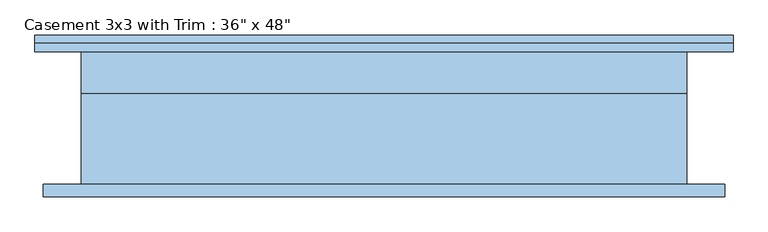
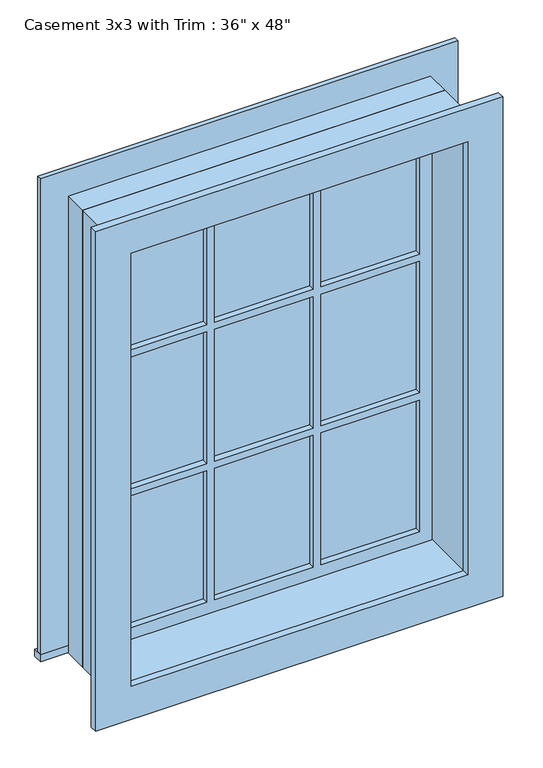
"""IFC4 building model written with IfcOpenShell, lengths in millimetres: window geometry."""

from ifc_helpers import new_model, si_unit, frame, origin, place, context, project, spatial, polyline, outline, extrude, source, transform, mapped, element, save


def window_ddc5d35f(model_context):
    return source(origin(), model_context, "Body", "SweptSolid", [
        extrude(outline(polyline([(-527.05, 125.4), (527.05, 125.4), (527.05, 100.0), (-527.05, 100.0), (-527.05, 125.4)])), frame((0.0, 0.0, 914.4), z_axis=(0.0, 0.0, 1.0), x_axis=(1.0, 0.0, 0.0)), (0.0, 0.0, 1.0), 19.05),
        extrude(outline(polyline([(2114.55, -438.15), (2114.55, 438.15), (933.45, 438.15), (933.45, 527.05), (2203.45, 527.05), (2203.45, -527.05), (933.45, -527.05), (933.45, -438.15), (2114.55, -438.15)])), frame((0.0, 100.0, 0.0), z_axis=(0.0, 1.0, 0.0), x_axis=(0.0, 0.0, 1.0)), (0.0, 0.0, 1.0), 12.7),
        extrude(outline(polyline([(143.9333333, 65.075), (393.7, 65.075), (393.7, 52.375), (143.9333333, 52.375), (143.9333333, 65.075)])), frame((0.0, 0.0, 1718.7333333), z_axis=(0.0, 0.0, 1.0), x_axis=(1.0, 0.0, 0.0)), (0.0, 0.0, 1.0), 351.3666667),
        extrude(outline(polyline([(-124.8833333, 65.075), (124.8833333, 65.075), (124.8833333, 52.375), (-124.8833333, 52.375), (-124.8833333, 65.075)])), frame((0.0, 0.0, 1718.7333333), z_axis=(0.0, 0.0, 1.0), x_axis=(1.0, 0.0, 0.0)), (0.0, 0.0, 1.0), 351.3666667),
        extrude(outline(polyline([(-393.7, 65.075), (-143.9333333, 65.075), (-143.9333333, 52.375), (-393.7, 52.375), (-393.7, 65.075)])), frame((0.0, 0.0, 1718.7333333), z_axis=(0.0, 0.0, 1.0), x_axis=(1.0, 0.0, 0.0)), (0.0, 0.0, 1.0), 351.3666667),
        extrude(outline(polyline([(-393.7, 65.075), (-143.9333333, 65.075), (-143.9333333, 52.375), (-393.7, 52.375), (-393.7, 65.075)])), frame((0.0, 0.0, 1348.3166667), z_axis=(0.0, 0.0, 1.0), x_axis=(1.0, 0.0, 0.0)), (0.0, 0.0, 1.0), 351.3666667),
        extrude(outline(polyline([(-124.8833333, 65.075), (124.8833333, 65.075), (124.8833333, 52.375), (-124.8833333, 52.375), (-124.8833333, 65.075)])), frame((0.0, 0.0, 1348.3166667), z_axis=(0.0, 0.0, 1.0), x_axis=(1.0, 0.0, 0.0)), (0.0, 0.0, 1.0), 351.3666667),
        extrude(outline(polyline([(143.9333333, 65.075), (393.7, 65.075), (393.7, 52.375), (143.9333333, 52.375), (143.9333333, 65.075)])), frame((0.0, 0.0, 1348.3166667), z_axis=(0.0, 0.0, 1.0), x_axis=(1.0, 0.0, 0.0)), (0.0, 0.0, 1.0), 351.3666667),
        extrude(outline(polyline([(143.9333333, 65.075), (393.7, 65.075), (393.7, 52.375), (143.9333333, 52.375), (143.9333333, 65.075)])), frame((0.0, 0.0, 977.9), z_axis=(0.0, 0.0, 1.0), x_axis=(1.0, 0.0, 0.0)), (0.0, 0.0, 1.0), 351.3666667),
        extrude(outline(polyline([(-124.8833333, 65.075), (124.8833333, 65.075), (124.8833333, 52.375), (-124.8833333, 52.375), (-124.8833333, 65.075)])), frame((0.0, 0.0, 977.9), z_axis=(0.0, 0.0, 1.0), x_axis=(1.0, 0.0, 0.0)), (0.0, 0.0, 1.0), 351.3666667),
        extrude(outline(polyline([(-393.7, 65.075), (-143.9333333, 65.075), (-143.9333333, 52.375), (-393.7, 52.375), (-393.7, 65.075)])), frame((0.0, 0.0, 977.9), z_axis=(0.0, 0.0, 1.0), x_axis=(1.0, 0.0, 0.0)), (0.0, 0.0, 1.0), 351.3666667),
        extrude(outline(polyline([(2190.75, 514.35), (2190.75, -514.35), (857.25, -514.35), (857.25, 514.35), (2190.75, 514.35)]), holes=[polyline([(2101.85, 425.45), (946.15, 425.45), (946.15, -425.45), (2101.85, -425.45), (2101.85, 425.45)])]), frame((0.0, -119.05, 0.0), z_axis=(0.0, 1.0, 0.0), x_axis=(0.0, 0.0, 1.0)), (0.0, 0.0, 1.0), 19.05),
        extrude(outline(polyline([(2114.55, -438.15), (933.45, -438.15), (933.45, 438.15), (2114.55, 438.15), (2114.55, -438.15)]), holes=[polyline([(2070.1, -143.9333333), (1718.7333333, -143.9333333), (1718.7333333, -393.7), (2070.1, -393.7), (2070.1, -143.9333333)]), polyline([(1699.6833333, -143.9333333), (1348.3166667, -143.9333333), (1348.3166667, -393.7), (1699.6833333, -393.7), (1699.6833333, -143.9333333)]), polyline([(1329.2666667, -143.9333333), (977.9, -143.9333333), (977.9, -393.7), (1329.2666667, -393.7), (1329.2666667, -143.9333333)]), polyline([(2070.1, 124.8833333), (1718.7333333, 124.8833333), (1718.7333333, -124.8833333), (2070.1, -124.8833333), (2070.1, 124.8833333)]), polyline([(1699.6833333, 124.8833333), (1348.3166667, 124.8833333), (1348.3166667, -124.8833333), (1699.6833333, -124.8833333), (1699.6833333, 124.8833333)]), polyline([(1329.2666667, 124.8833333), (977.9, 124.8833333), (977.9, -124.8833333), (1329.2666667, -124.8833333), (1329.2666667, 124.8833333)]), polyline([(2070.1, 393.7), (1718.7333333, 393.7), (1718.7333333, 143.9333333), (2070.1, 143.9333333), (2070.1, 393.7)]), polyline([(1699.6833333, 393.7), (1348.3166667, 393.7), (1348.3166667, 143.9333333), (1699.6833333, 143.9333333), (1699.6833333, 393.7)]), polyline([(1329.2666667, 393.7), (977.9, 393.7), (977.9, 143.9333333), (1329.2666667, 143.9333333), (1329.2666667, 393.7)])]), frame((0.0, 36.5, 0.0), z_axis=(0.0, 1.0, 0.0), x_axis=(0.0, 0.0, 1.0)), (0.0, 0.0, 1.0), 44.45),
        extrude(outline(polyline([(2133.6, -457.2), (914.4, -457.2), (914.4, 457.2), (2133.6, 457.2), (2133.6, -457.2)]), holes=[polyline([(2101.85, -425.45), (2101.85, 425.45), (946.15, 425.45), (946.15, -425.45), (2101.85, -425.45)])]), frame((0.0, -100.0, 0.0), z_axis=(0.0, 1.0, 0.0), x_axis=(0.0, 0.0, 1.0)), (0.0, 0.0, 1.0), 136.5),
        extrude(outline(polyline([(2133.6, 457.2), (2133.6, -457.2), (914.4, -457.2), (914.4, 457.2), (2133.6, 457.2)]), holes=[polyline([(2114.55, 438.15), (933.45, 438.15), (933.45, -438.15), (2114.55, -438.15), (2114.55, 438.15)])]), frame((0.0, 36.5, 0.0), z_axis=(0.0, 1.0, 0.0), x_axis=(0.0, 0.0, 1.0)), (0.0, 0.0, 1.0), 63.5),
    ])


if __name__ == "__main__":
    model = new_model("IFC4")
    model_context = context("Model", 3, world=origin())
    ifc_project = project(units=[si_unit("LENGTHUNIT", "METRE", prefix="MILLI")], contexts=[model_context])
    site = spatial("IfcSite", under=ifc_project)
    building = spatial("IfcBuilding", under=site)
    placement = place(None, origin())
    window_shape = window_ddc5d35f(model_context)
    element("IfcWindow", 1, ObjectType="Casement 3x3 with Trim : 36\" x 48\"", at=placement, inside=building, context=model_context, shape_type="MappedRepresentation", body=[
        mapped(window_shape, transform((0.0, 0.0, 0.0), x_axis=(1.0, 0.0, 0.0), y_axis=(0.0, 1.0, 0.0), z_axis=(0.0, 0.0, 1.0))),
    ])
    save(model, "model.ifc")

# Revit data of these elements
# Type "Casement 3x3 with Trim : 36\" x 48\""
#   Type Mark = "25"
#   Construction Type Id = "GSP4R"
#   Assembly Code = "B2020100"
#   Analytic Construction = "1/8 in Pilkington single glazing"
#   Visual Light Transmittance = 0.9
#   Solar Heat Gain Coefficient = 0.78
#   Heat Transfer Coefficient (U) = 3.6886 W/(m²·K)
#   Height = 4' - 0"
#   Default Sill Height = 3' - 0"
#   Trim Projection - Ext. = 0' - 0 1/2"
#   Trim Projection - Int. = 0' - 0 3/4"
#   Trim Width - Exterior = 0' - 3 1/2"
#   Trim Width - Interior = 0' - 3 1/2"
#   Width = 3' - 0"
#   Window Inset = 0' - 0 3/4"
#   Define Thermal Properties by = 1
#   Glass Pane Material = Glass
#   Sash Material = Sash
#   Trim Exterior Material = Trim
#   Trim Interior Material = Trim
#   Wall Closure = (empty or 0)
# Element 1 (IfcWindow, "Casement 3x3 with Trim : 36\" x 48\"")
#   Materials on its faces: "Sash", "Glass", "Trim"
# Materials
#   "Glass": class "Glass", colour RGB 218 227 224, transparency 0.85, Description = "Soda Lime Glass", Cost = 0
#   "Sash": class "Wood", colour RGB 136 99 55, transparency 0
#   "Trim": class "Wood", colour RGB 224 178 126, transparency 0
